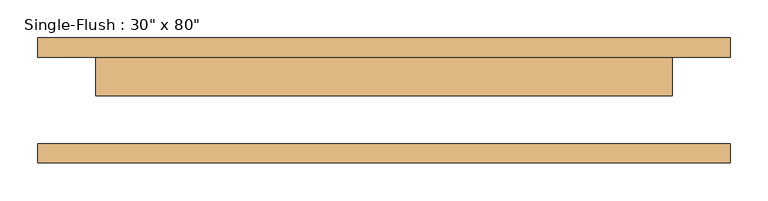
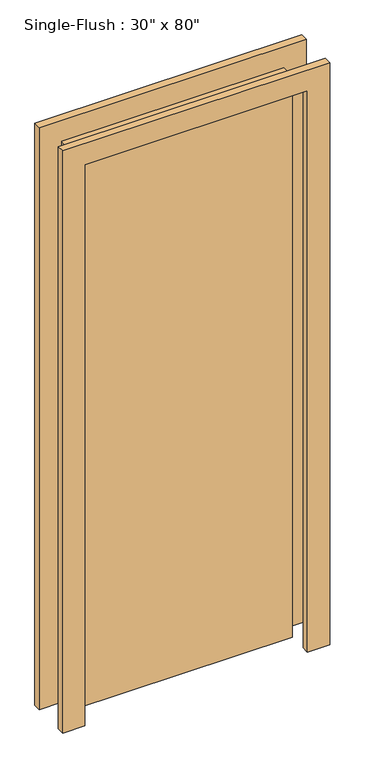
"""IFC4 building model written with IfcOpenShell, lengths in millimetres: door geometry."""

from ifc_helpers import new_model, si_unit, frame, origin, origin_with_axes, place, context, project, spatial, polyline, outline, extrude, source, transform, mapped, element, save


def door_d8f5dbb5(model_context):
    return source(origin(), model_context, "Body", "SweptSolid", [
        extrude(outline(polyline([(2108.2, -457.2), (0.0, -457.2), (0.0, -381.0), (2032.0, -381.0), (2032.0, 381.0), (0.0, 381.0), (0.0, 457.2), (2108.2, 457.2), (2108.2, -457.2)])), frame((0.0, 57.15, 0.0), z_axis=(0.0, 1.0, 0.0), x_axis=(0.0, 0.0, 1.0)), (0.0, 0.0, 1.0), 25.4),
        extrude(outline(polyline([(2108.2, 457.2), (2108.2, -457.2), (0.0, -457.2), (0.0, -381.0), (2032.0, -381.0), (2032.0, 381.0), (0.0, 381.0), (0.0, 457.2), (2108.2, 457.2)])), frame((0.0, -82.55, 0.0), z_axis=(0.0, 1.0, 0.0), x_axis=(0.0, 0.0, 1.0)), (0.0, 0.0, 1.0), 25.4),
        extrude(outline(polyline([(381.0, 6.35), (-381.0, 6.35), (-381.0, 57.15), (381.0, 57.15), (381.0, 6.35)])), origin_with_axes(), (0.0, 0.0, 1.0), 2032.0),
    ])


if __name__ == "__main__":
    model = new_model("IFC4")
    model_context = context("Model", 3, world=origin())
    ifc_project = project(units=[si_unit("LENGTHUNIT", "METRE", prefix="MILLI")], contexts=[model_context])
    site = spatial("IfcSite", under=ifc_project)
    building = spatial("IfcBuilding", under=site)
    placement = place(None, origin())
    door_shape = door_d8f5dbb5(model_context)
    element("IfcDoor", 1, ObjectType="Single-Flush : 30\" x 80\"", at=placement, inside=building, context=model_context, shape_type="MappedRepresentation", body=[
        mapped(door_shape, transform((0.0, 0.0, 0.0), x_axis=(1.0, 0.0, 0.0), y_axis=(0.0, 1.0, 0.0), z_axis=(0.0, 0.0, 1.0))),
    ])
    save(model, "model.ifc")

# Revit data of these elements
# Type "Single-Flush : 30\" x 80\""
#   Type Mark = "12"
#   Construction Type Id = "MDOOR"
#   Assembly Code = "C1020"
#   Analytic Construction = "Metal"
#   Thickness = 0' - 2"
#   Heat Transfer Coefficient (U) = 0.651978 BTU/(h·ft²·°F)
#   Height = 6' - 8"
#   Trim Projection Ext = 0' - 1"
#   Trim Projection Int = 0' - 1"
#   Trim Width = 0' - 3"
#   Width = 2' - 6"
#   Define Thermal Properties by = 1
#   Define Thermal Properties by = 1
#   Door Material = Door - Panel
#   Frame Material = Door - Frame
#   Visual Light Transmittance = 0
#   Solar Heat Gain Coefficient = 0
#   Function = (empty or 0)
#   Wall Closure = (empty or 0)
# Element 1 (IfcDoor, "Single-Flush : 30\" x 80\"")
#   Materials on its faces: "Door - Frame", "Door - Panel"
# Materials
#   "Door - Panel": class "Wood", colour RGB 210 159 95, transparency 0, Cost = 0
#   "Door - Frame": colour RGB 118 70 51, transparency 0, Cost = 0
